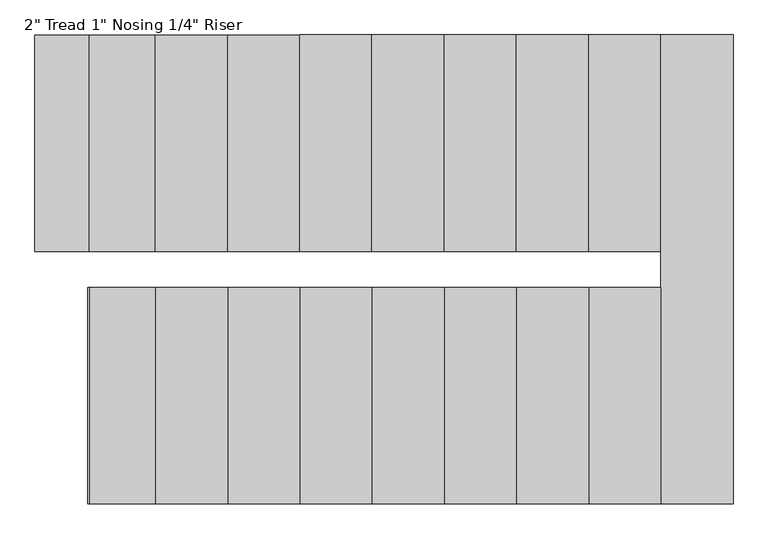
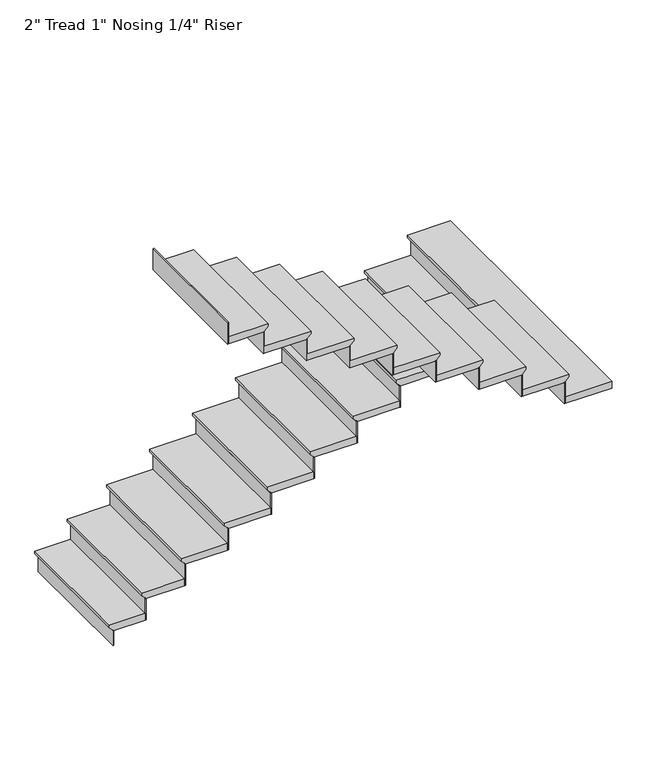
"""IFC4 building model written with IfcOpenShell, lengths in millimetres: stair flight geometry."""

from ifc_helpers import new_model, si_unit, origin, place, context, project, spatial, faceted_brep, source, transform, mapped, element, save


def stair_flight_3d163d7c(model_context):
    return source(origin(), model_context, "Body", "Brep", [
        faceted_brep([(8572.5, 8280.4, 3189.3710526), (8572.5, 8280.4, 3208.4210526), (8572.5, 9194.8, 3208.4210526), (8572.5, 9194.8, 3189.3710526), (8597.9, 8280.4, 3163.9710526), (8597.9, 9194.8, 3163.9710526), (8826.5, 8280.4, 3208.4210526), (8826.5, 9194.8, 3208.4210526), (8597.9, 9194.8, 3157.6210526), (8826.5, 9194.8, 3157.6210526), (8826.5, 8280.4, 3157.6210526), (8597.9, 8280.4, 3157.6210526)], [[[0, 1, 2, 3]], [[4, 0, 3, 5]], [[2, 1, 6, 7]], [[8, 9, 10, 11]], [[2, 7, 9, 8, 5, 3]], [[8, 11, 4, 5]], [[6, 1, 0, 4, 11, 10]], [[7, 6, 10, 9]]]),
        faceted_brep([(8597.9, 8280.4, 3157.6210526), (8597.9, 8280.4, 3048.0), (8604.25, 8280.4, 3048.0), (8604.25, 8280.4, 3157.6210526), (8597.9, 9194.8, 3157.6210526), (8604.25, 9194.8, 3157.6210526), (8604.25, 9194.8, 3048.0), (8597.9, 9194.8, 3048.0)], [[[0, 1, 2, 3]], [[4, 5, 6, 7]], [[1, 0, 4, 7]], [[2, 1, 7, 6]], [[3, 2, 6, 5]], [[0, 3, 5, 4]]]),
        faceted_brep([(8826.5, 8280.4, 3318.0421053), (8826.5, 8280.4, 3157.6210526), (8832.85, 8280.4, 3157.6210526), (8832.85, 8280.4, 3318.0421053), (8826.5, 9194.8, 3318.0421053), (8832.85, 9194.8, 3318.0421053), (8832.85, 9194.8, 3157.6210526), (8826.5, 9194.8, 3157.6210526)], [[[0, 1, 2, 3]], [[4, 5, 6, 7]], [[1, 0, 4, 7]], [[2, 1, 7, 6]], [[3, 2, 6, 5]], [[0, 3, 5, 4]]]),
        faceted_brep([(8801.1, 9194.8, 3368.8421053), (8801.1, 8280.4, 3368.8421053), (9105.9, 8280.4, 3368.8421053), (9105.9, 9194.8, 3368.8421053), (8826.5, 9194.8, 3318.0421053), (9105.9, 9194.8, 3318.0421053), (9105.9, 8280.4, 3318.0421053), (8826.5, 8280.4, 3318.0421053), (8826.5, 9194.8, 3324.3921053), (8801.1, 9194.8, 3349.7921053), (8826.5, 8280.4, 3324.3921053), (8801.1, 8280.4, 3349.7921053)], [[[0, 1, 2, 3]], [[4, 5, 6, 7]], [[0, 3, 5, 4, 8, 9]], [[4, 7, 10, 8]], [[2, 1, 11, 10, 7, 6]], [[3, 2, 6, 5]], [[11, 1, 0, 9]], [[10, 11, 9, 8]]]),
        faceted_brep([(9105.9, 8280.4, 3478.4631579), (9105.9, 8280.4, 3318.0421053), (9112.25, 8280.4, 3318.0421053), (9112.25, 8280.4, 3478.4631579), (9105.9, 9194.8, 3478.4631579), (9112.25, 9194.8, 3478.4631579), (9112.25, 9194.8, 3318.0421053), (9105.9, 9194.8, 3318.0421053)], [[[0, 1, 2, 3]], [[4, 5, 6, 7]], [[1, 0, 4, 7]], [[2, 1, 7, 6]], [[3, 2, 6, 5]], [[0, 3, 5, 4]]]),
        faceted_brep([(9080.5, 9194.8, 3529.2631579), (9080.5, 8280.4, 3529.2631579), (9410.7, 8280.4, 3529.2631579), (9410.7, 9194.8, 3529.2631579), (9105.9, 9194.8, 3478.4631579), (9410.7, 9194.8, 3478.4631579), (9410.7, 8280.4, 3478.4631579), (9105.9, 8280.4, 3478.4631579), (9105.9, 9194.8, 3484.8131579), (9080.5, 9194.8, 3510.2131579), (9105.9, 8280.4, 3484.8131579), (9080.5, 8280.4, 3510.2131579)], [[[0, 1, 2, 3]], [[4, 5, 6, 7]], [[0, 3, 5, 4, 8, 9]], [[4, 7, 10, 8]], [[2, 1, 11, 10, 7, 6]], [[3, 2, 6, 5]], [[11, 1, 0, 9]], [[10, 11, 9, 8]]]),
        faceted_brep([(9410.7, 8280.4, 3638.8842105), (9410.7, 8280.4, 3478.4631579), (9417.05, 8280.4, 3478.4631579), (9417.05, 8280.4, 3638.8842105), (9410.7, 9194.8, 3638.8842105), (9417.05, 9194.8, 3638.8842105), (9417.05, 9194.8, 3478.4631579), (9410.7, 9194.8, 3478.4631579)], [[[0, 1, 2, 3]], [[4, 5, 6, 7]], [[1, 0, 4, 7]], [[2, 1, 7, 6]], [[3, 2, 6, 5]], [[0, 3, 5, 4]]]),
        faceted_brep([(9385.3, 9194.8, 3689.6842105), (9385.3, 8280.4, 3689.6842105), (9715.5, 8280.4, 3689.6842105), (9715.5, 9194.8, 3689.6842105), (9410.7, 9194.8, 3638.8842105), (9715.5, 9194.8, 3638.8842105), (9715.5, 8280.4, 3638.8842105), (9410.7, 8280.4, 3638.8842105), (9410.7, 9194.8, 3645.2342105), (9385.3, 9194.8, 3670.6342105), (9410.7, 8280.4, 3645.2342105), (9385.3, 8280.4, 3670.6342105)], [[[0, 1, 2, 3]], [[4, 5, 6, 7]], [[0, 3, 5, 4, 8, 9]], [[4, 7, 10, 8]], [[2, 1, 11, 10, 7, 6]], [[3, 2, 6, 5]], [[11, 1, 0, 9]], [[10, 11, 9, 8]]]),
        faceted_brep([(9715.5, 8280.4, 3799.3052632), (9715.5, 8280.4, 3638.8842105), (9721.85, 8280.4, 3638.8842105), (9721.85, 8280.4, 3799.3052632), (9715.5, 9194.8, 3799.3052632), (9721.85, 9194.8, 3799.3052632), (9721.85, 9194.8, 3638.8842105), (9715.5, 9194.8, 3638.8842105)], [[[0, 1, 2, 3]], [[4, 5, 6, 7]], [[1, 0, 4, 7]], [[2, 1, 7, 6]], [[3, 2, 6, 5]], [[0, 3, 5, 4]]]),
        faceted_brep([(9690.1, 9194.8, 3850.1052632), (9690.1, 8280.4, 3850.1052632), (10020.3, 8280.4, 3850.1052632), (10020.3, 9194.8, 3850.1052632), (9715.5, 9194.8, 3799.3052632), (10020.3, 9194.8, 3799.3052632), (10020.3, 8280.4, 3799.3052632), (9715.5, 8280.4, 3799.3052632), (9715.5, 9194.8, 3805.6552632), (9690.1, 9194.8, 3831.0552632), (9715.5, 8280.4, 3805.6552632), (9690.1, 8280.4, 3831.0552632)], [[[0, 1, 2, 3]], [[4, 5, 6, 7]], [[0, 3, 5, 4, 8, 9]], [[4, 7, 10, 8]], [[2, 1, 11, 10, 7, 6]], [[3, 2, 6, 5]], [[11, 1, 0, 9]], [[10, 11, 9, 8]]]),
        faceted_brep([(10020.3, 8280.4, 3959.7263158), (10020.3, 8280.4, 3799.3052632), (10026.65, 8280.4, 3799.3052632), (10026.65, 8280.4, 3959.7263158), (10020.3, 9194.8, 3959.7263158), (10026.65, 9194.8, 3959.7263158), (10026.65, 9194.8, 3799.3052632), (10020.3, 9194.8, 3799.3052632)], [[[0, 1, 2, 3]], [[4, 5, 6, 7]], [[1, 0, 4, 7]], [[2, 1, 7, 6]], [[3, 2, 6, 5]], [[0, 3, 5, 4]]]),
        faceted_brep([(9994.9, 9194.8, 4010.5263158), (9994.9, 8280.4, 4010.5263158), (10325.1, 8280.4, 4010.5263158), (10325.1, 9194.8, 4010.5263158), (10020.3, 9194.8, 3959.7263158), (10325.1, 9194.8, 3959.7263158), (10325.1, 8280.4, 3959.7263158), (10020.3, 8280.4, 3959.7263158), (10020.3, 9194.8, 3966.0763158), (9994.9, 9194.8, 3991.4763158), (10020.3, 8280.4, 3966.0763158), (9994.9, 8280.4, 3991.4763158)], [[[0, 1, 2, 3]], [[4, 5, 6, 7]], [[0, 3, 5, 4, 8, 9]], [[4, 7, 10, 8]], [[2, 1, 11, 10, 7, 6]], [[3, 2, 6, 5]], [[11, 1, 0, 9]], [[10, 11, 9, 8]]]),
        faceted_brep([(10325.1, 8280.4, 4120.1473684), (10325.1, 8280.4, 3959.7263158), (10331.45, 8280.4, 3959.7263158), (10331.45, 8280.4, 4120.1473684), (10325.1, 9194.8, 4120.1473684), (10331.45, 9194.8, 4120.1473684), (10331.45, 9194.8, 3959.7263158), (10325.1, 9194.8, 3959.7263158)], [[[0, 1, 2, 3]], [[4, 5, 6, 7]], [[1, 0, 4, 7]], [[2, 1, 7, 6]], [[3, 2, 6, 5]], [[0, 3, 5, 4]]]),
        faceted_brep([(10299.7, 9194.8, 4170.9473684), (10299.7, 8280.4, 4170.9473684), (10629.9, 8280.4, 4170.9473684), (10629.9, 9194.8, 4170.9473684), (10325.1, 9194.8, 4120.1473684), (10629.9, 9194.8, 4120.1473684), (10629.9, 8280.4, 4120.1473684), (10325.1, 8280.4, 4120.1473684), (10325.1, 9194.8, 4126.4973684), (10299.7, 9194.8, 4151.8973684), (10325.1, 8280.4, 4126.4973684), (10299.7, 8280.4, 4151.8973684)], [[[0, 1, 2, 3]], [[4, 5, 6, 7]], [[0, 3, 5, 4, 8, 9]], [[4, 7, 10, 8]], [[2, 1, 11, 10, 7, 6]], [[3, 2, 6, 5]], [[11, 1, 0, 9]], [[10, 11, 9, 8]]]),
        faceted_brep([(10629.9, 8280.4, 4280.5684211), (10629.9, 8280.4, 4120.1473684), (10636.25, 8280.4, 4120.1473684), (10636.25, 8280.4, 4280.5684211), (10629.9, 9194.8, 4280.5684211), (10636.25, 9194.8, 4280.5684211), (10636.25, 9194.8, 4120.1473684), (10629.9, 9194.8, 4120.1473684)], [[[0, 1, 2, 3]], [[4, 5, 6, 7]], [[1, 0, 4, 7]], [[2, 1, 7, 6]], [[3, 2, 6, 5]], [[0, 3, 5, 4]]]),
        faceted_brep([(10604.5, 9194.8, 4331.3684211), (10604.5, 8280.4, 4331.3684211), (10934.7, 8280.4, 4331.3684211), (10934.7, 9194.8, 4331.3684211), (10629.9, 9194.8, 4280.5684211), (10934.7, 9194.8, 4280.5684211), (10934.7, 8280.4, 4280.5684211), (10629.9, 8280.4, 4280.5684211), (10629.9, 9194.8, 4286.9184211), (10604.5, 9194.8, 4312.3184211), (10629.9, 8280.4, 4286.9184211), (10604.5, 8280.4, 4312.3184211)], [[[0, 1, 2, 3]], [[4, 5, 6, 7]], [[0, 3, 5, 4, 8, 9]], [[4, 7, 10, 8]], [[2, 1, 11, 10, 7, 6]], [[3, 2, 6, 5]], [[11, 1, 0, 9]], [[10, 11, 9, 8]]]),
        faceted_brep([(10934.7, 8280.4, 4440.9894737), (10934.7, 8280.4, 4280.5684211), (10941.05, 8280.4, 4280.5684211), (10941.05, 8280.4, 4440.9894737), (10934.7, 9194.8, 4440.9894737), (10941.05, 9194.8, 4440.9894737), (10941.05, 9194.8, 4280.5684211), (10934.7, 9194.8, 4280.5684211)], [[[0, 1, 2, 3]], [[4, 5, 6, 7]], [[1, 0, 4, 7]], [[2, 1, 7, 6]], [[3, 2, 6, 5]], [[0, 3, 5, 4]]]),
        faceted_brep([(10909.3, 9194.8, 4491.7894737), (10909.3, 8280.4, 4491.7894737), (11239.5, 8280.4, 4491.7894737), (11239.5, 9194.8, 4491.7894737), (10934.7, 9194.8, 4440.9894737), (11239.5, 9194.8, 4440.9894737), (11239.5, 8280.4, 4440.9894737), (10934.7, 8280.4, 4440.9894737), (10934.7, 9194.8, 4447.3394737), (10909.3, 9194.8, 4472.7394737), (10934.7, 8280.4, 4447.3394737), (10909.3, 8280.4, 4472.7394737)], [[[0, 1, 2, 3]], [[4, 5, 6, 7]], [[0, 3, 5, 4, 8, 9]], [[4, 7, 10, 8]], [[2, 1, 11, 10, 7, 6]], [[3, 2, 6, 5]], [[11, 1, 0, 9]], [[10, 11, 9, 8]]]),
        faceted_brep([(11239.5, 8280.4, 4601.4105263), (11239.5, 8280.4, 4440.9894737), (11245.85, 8280.4, 4440.9894737), (11245.85, 8280.4, 4601.4105263), (11239.5, 9194.8, 4601.4105263), (11245.85, 9194.8, 4601.4105263), (11245.85, 9194.8, 4440.9894737), (11239.5, 9194.8, 4440.9894737)], [[[0, 1, 2, 3]], [[4, 5, 6, 7]], [[1, 0, 4, 7]], [[2, 1, 7, 6]], [[3, 2, 6, 5]], [[0, 3, 5, 4]]]),
        faceted_brep([(11188.7, 7213.6, 4652.2105263), (11518.9, 7213.6, 4652.2105263), (11518.9, 9194.8, 4652.2105263), (11214.1, 9194.8, 4652.2105263), (11214.1, 8128.0, 4652.2105263), (11188.7, 8128.0, 4652.2105263), (11518.9, 7213.6, 4601.4105263), (11188.7, 7213.6, 4601.4105263), (11188.7, 8128.0, 4601.4105263), (11214.1, 8128.0, 4601.4105263), (11214.1, 8280.4, 4601.4105263), (11239.5, 8280.4, 4601.4105263), (11239.5, 9194.8, 4601.4105263), (11518.9, 9194.8, 4601.4105263), (11239.5, 9194.8, 4607.7605263), (11214.1, 9194.8, 4633.1605263), (11239.5, 8280.4, 4607.7605263), (11214.1, 8280.4, 4633.1605263)], [[[0, 1, 2, 3, 4, 5]], [[6, 7, 8, 9, 10, 11, 12, 13]], [[1, 0, 7, 6]], [[2, 1, 6, 13]], [[3, 2, 13, 12, 14, 15]], [[12, 11, 16, 14]], [[11, 10, 17, 16]], [[4, 3, 15, 17, 10, 9]], [[5, 4, 9, 8]], [[0, 5, 8, 7]], [[15, 14, 16, 17]]]),
        faceted_brep([(11188.7, 8128.0, 4761.8315789), (11188.7, 8128.0, 4601.4105263), (11182.35, 8128.0, 4601.4105263), (11182.35, 8128.0, 4761.8315789), (11188.7, 7213.6, 4761.8315789), (11182.35, 7213.6, 4761.8315789), (11182.35, 7213.6, 4601.4105263), (11188.7, 7213.6, 4601.4105263)], [[[0, 1, 2, 3]], [[4, 5, 6, 7]], [[1, 0, 4, 7]], [[2, 1, 7, 6]], [[3, 2, 6, 5]], [[0, 3, 5, 4]]]),
        faceted_brep([(11214.1, 7213.6, 4812.6315789), (11214.1, 8128.0, 4812.6315789), (10883.9, 8128.0, 4812.6315789), (10883.9, 7213.6, 4812.6315789), (11188.7, 7213.6, 4761.8315789), (10883.9, 7213.6, 4761.8315789), (10883.9, 8128.0, 4761.8315789), (11188.7, 8128.0, 4761.8315789), (11188.7, 7213.6, 4768.1815789), (11214.1, 7213.6, 4793.5815789), (11188.7, 8128.0, 4768.1815789), (11214.1, 8128.0, 4793.5815789)], [[[0, 1, 2, 3]], [[4, 5, 6, 7]], [[0, 3, 5, 4, 8, 9]], [[4, 7, 10, 8]], [[2, 1, 11, 10, 7, 6]], [[3, 2, 6, 5]], [[11, 1, 0, 9]], [[10, 11, 9, 8]]]),
        faceted_brep([(10883.9, 8128.0, 4922.2526316), (10883.9, 8128.0, 4761.8315789), (10877.55, 8128.0, 4761.8315789), (10877.55, 8128.0, 4922.2526316), (10883.9, 7213.6, 4922.2526316), (10877.55, 7213.6, 4922.2526316), (10877.55, 7213.6, 4761.8315789), (10883.9, 7213.6, 4761.8315789)], [[[0, 1, 2, 3]], [[4, 5, 6, 7]], [[1, 0, 4, 7]], [[2, 1, 7, 6]], [[3, 2, 6, 5]], [[0, 3, 5, 4]]]),
        faceted_brep([(10909.3, 7213.6, 4973.0526316), (10909.3, 8128.0, 4973.0526316), (10579.1, 8128.0, 4973.0526316), (10579.1, 7213.6, 4973.0526316), (10883.9, 7213.6, 4922.2526316), (10579.1, 7213.6, 4922.2526316), (10579.1, 8128.0, 4922.2526316), (10883.9, 8128.0, 4922.2526316), (10883.9, 7213.6, 4928.6026316), (10909.3, 7213.6, 4954.0026316), (10883.9, 8128.0, 4928.6026316), (10909.3, 8128.0, 4954.0026316)], [[[0, 1, 2, 3]], [[4, 5, 6, 7]], [[0, 3, 5, 4, 8, 9]], [[4, 7, 10, 8]], [[2, 1, 11, 10, 7, 6]], [[3, 2, 6, 5]], [[11, 1, 0, 9]], [[10, 11, 9, 8]]]),
        faceted_brep([(10579.1, 8128.0, 5082.6736842), (10579.1, 8128.0, 4922.2526316), (10572.75, 8128.0, 4922.2526316), (10572.75, 8128.0, 5082.6736842), (10579.1, 7213.6, 5082.6736842), (10572.75, 7213.6, 5082.6736842), (10572.75, 7213.6, 4922.2526316), (10579.1, 7213.6, 4922.2526316)], [[[0, 1, 2, 3]], [[4, 5, 6, 7]], [[1, 0, 4, 7]], [[2, 1, 7, 6]], [[3, 2, 6, 5]], [[0, 3, 5, 4]]]),
        faceted_brep([(10604.5, 7213.6, 5133.4736842), (10604.5, 8128.0, 5133.4736842), (10274.3, 8128.0, 5133.4736842), (10274.3, 7213.6, 5133.4736842), (10579.1, 7213.6, 5082.6736842), (10274.3, 7213.6, 5082.6736842), (10274.3, 8128.0, 5082.6736842), (10579.1, 8128.0, 5082.6736842), (10579.1, 7213.6, 5089.0236842), (10604.5, 7213.6, 5114.4236842), (10579.1, 8128.0, 5089.0236842), (10604.5, 8128.0, 5114.4236842)], [[[0, 1, 2, 3]], [[4, 5, 6, 7]], [[0, 3, 5, 4, 8, 9]], [[4, 7, 10, 8]], [[2, 1, 11, 10, 7, 6]], [[3, 2, 6, 5]], [[11, 1, 0, 9]], [[10, 11, 9, 8]]]),
        faceted_brep([(10274.3, 8128.0, 5243.0947368), (10274.3, 8128.0, 5082.6736842), (10267.95, 8128.0, 5082.6736842), (10267.95, 8128.0, 5243.0947368), (10274.3, 7213.6, 5243.0947368), (10267.95, 7213.6, 5243.0947368), (10267.95, 7213.6, 5082.6736842), (10274.3, 7213.6, 5082.6736842)], [[[0, 1, 2, 3]], [[4, 5, 6, 7]], [[1, 0, 4, 7]], [[2, 1, 7, 6]], [[3, 2, 6, 5]], [[0, 3, 5, 4]]]),
        faceted_brep([(10299.7, 7213.6, 5293.8947368), (10299.7, 8128.0, 5293.8947368), (9969.5, 8128.0, 5293.8947368), (9969.5, 7213.6, 5293.8947368), (10274.3, 7213.6, 5243.0947368), (9969.5, 7213.6, 5243.0947368), (9969.5, 8128.0, 5243.0947368), (10274.3, 8128.0, 5243.0947368), (10274.3, 7213.6, 5249.4447368), (10299.7, 7213.6, 5274.8447368), (10274.3, 8128.0, 5249.4447368), (10299.7, 8128.0, 5274.8447368)], [[[0, 1, 2, 3]], [[4, 5, 6, 7]], [[0, 3, 5, 4, 8, 9]], [[4, 7, 10, 8]], [[2, 1, 11, 10, 7, 6]], [[3, 2, 6, 5]], [[11, 1, 0, 9]], [[10, 11, 9, 8]]]),
        faceted_brep([(9969.5, 8128.0, 5403.5157895), (9969.5, 8128.0, 5243.0947368), (9963.15, 8128.0, 5243.0947368), (9963.15, 8128.0, 5403.5157895), (9969.5, 7213.6, 5403.5157895), (9963.15, 7213.6, 5403.5157895), (9963.15, 7213.6, 5243.0947368), (9969.5, 7213.6, 5243.0947368)], [[[0, 1, 2, 3]], [[4, 5, 6, 7]], [[1, 0, 4, 7]], [[2, 1, 7, 6]], [[3, 2, 6, 5]], [[0, 3, 5, 4]]]),
        faceted_brep([(9994.9, 7213.6, 5454.3157895), (9994.9, 8128.0, 5454.3157895), (9664.7, 8128.0, 5454.3157895), (9664.7, 7213.6, 5454.3157895), (9969.5, 7213.6, 5403.5157895), (9664.7, 7213.6, 5403.5157895), (9664.7, 8128.0, 5403.5157895), (9969.5, 8128.0, 5403.5157895), (9969.5, 7213.6, 5409.8657895), (9994.9, 7213.6, 5435.2657895), (9969.5, 8128.0, 5409.8657895), (9994.9, 8128.0, 5435.2657895)], [[[0, 1, 2, 3]], [[4, 5, 6, 7]], [[0, 3, 5, 4, 8, 9]], [[4, 7, 10, 8]], [[2, 1, 11, 10, 7, 6]], [[3, 2, 6, 5]], [[11, 1, 0, 9]], [[10, 11, 9, 8]]]),
        faceted_brep([(9664.7, 8128.0, 5563.9368421), (9664.7, 8128.0, 5403.5157895), (9658.35, 8128.0, 5403.5157895), (9658.35, 8128.0, 5563.9368421), (9664.7, 7213.6, 5563.9368421), (9658.35, 7213.6, 5563.9368421), (9658.35, 7213.6, 5403.5157895), (9664.7, 7213.6, 5403.5157895)], [[[0, 1, 2, 3]], [[4, 5, 6, 7]], [[1, 0, 4, 7]], [[2, 1, 7, 6]], [[3, 2, 6, 5]], [[0, 3, 5, 4]]]),
        faceted_brep([(9690.1, 7213.6, 5614.7368421), (9690.1, 8128.0, 5614.7368421), (9359.9, 8128.0, 5614.7368421), (9359.9, 7213.6, 5614.7368421), (9664.7, 7213.6, 5563.9368421), (9359.9, 7213.6, 5563.9368421), (9359.9, 8128.0, 5563.9368421), (9664.7, 8128.0, 5563.9368421), (9664.7, 7213.6, 5570.2868421), (9690.1, 7213.6, 5595.6868421), (9664.7, 8128.0, 5570.2868421), (9690.1, 8128.0, 5595.6868421)], [[[0, 1, 2, 3]], [[4, 5, 6, 7]], [[0, 3, 5, 4, 8, 9]], [[4, 7, 10, 8]], [[2, 1, 11, 10, 7, 6]], [[3, 2, 6, 5]], [[11, 1, 0, 9]], [[10, 11, 9, 8]]]),
        faceted_brep([(9359.9, 8128.0, 5724.3578947), (9359.9, 8128.0, 5563.9368421), (9353.55, 8128.0, 5563.9368421), (9353.55, 8128.0, 5724.3578947), (9359.9, 7213.6, 5724.3578947), (9353.55, 7213.6, 5724.3578947), (9353.55, 7213.6, 5563.9368421), (9359.9, 7213.6, 5563.9368421)], [[[0, 1, 2, 3]], [[4, 5, 6, 7]], [[1, 0, 4, 7]], [[2, 1, 7, 6]], [[3, 2, 6, 5]], [[0, 3, 5, 4]]]),
        faceted_brep([(9385.3, 7213.6, 5775.1578947), (9385.3, 8128.0, 5775.1578947), (9055.1, 8128.0, 5775.1578947), (9055.1, 7213.6, 5775.1578947), (9359.9, 7213.6, 5724.3578947), (9055.1, 7213.6, 5724.3578947), (9055.1, 8128.0, 5724.3578947), (9359.9, 8128.0, 5724.3578947), (9359.9, 7213.6, 5730.7078947), (9385.3, 7213.6, 5756.1078947), (9359.9, 8128.0, 5730.7078947), (9385.3, 8128.0, 5756.1078947)], [[[0, 1, 2, 3]], [[4, 5, 6, 7]], [[0, 3, 5, 4, 8, 9]], [[4, 7, 10, 8]], [[2, 1, 11, 10, 7, 6]], [[3, 2, 6, 5]], [[11, 1, 0, 9]], [[10, 11, 9, 8]]]),
        faceted_brep([(9055.1, 8128.0, 5884.7789474), (9055.1, 8128.0, 5724.3578947), (9048.75, 8128.0, 5724.3578947), (9048.75, 8128.0, 5884.7789474), (9055.1, 7213.6, 5884.7789474), (9048.75, 7213.6, 5884.7789474), (9048.75, 7213.6, 5724.3578947), (9055.1, 7213.6, 5724.3578947)], [[[0, 1, 2, 3]], [[4, 5, 6, 7]], [[1, 0, 4, 7]], [[2, 1, 7, 6]], [[3, 2, 6, 5]], [[0, 3, 5, 4]]]),
        faceted_brep([(8801.1, 8128.0, 6045.2), (8801.1, 8128.0, 5884.7789474), (8794.75, 8128.0, 5884.7789474), (8794.75, 8128.0, 6045.2), (8801.1, 7213.6, 6045.2), (8794.75, 7213.6, 6045.2), (8794.75, 7213.6, 5884.7789474), (8801.1, 7213.6, 5884.7789474)], [[[0, 1, 2, 3]], [[4, 5, 6, 7]], [[1, 0, 4, 7]], [[2, 1, 7, 6]], [[3, 2, 6, 5]], [[0, 3, 5, 4]]]),
        faceted_brep([(9080.5, 7213.6, 5935.5789474), (9080.5, 8128.0, 5935.5789474), (8801.1, 8128.0, 5935.5789474), (8801.1, 7213.6, 5935.5789474), (9055.1, 7213.6, 5884.7789474), (8801.1, 7213.6, 5884.7789474), (8801.1, 8128.0, 5884.7789474), (9055.1, 8128.0, 5884.7789474), (9055.1, 7213.6, 5891.1289474), (9080.5, 7213.6, 5916.5289474), (9055.1, 8128.0, 5891.1289474), (9080.5, 8128.0, 5916.5289474)], [[[0, 1, 2, 3]], [[4, 5, 6, 7]], [[0, 3, 5, 4, 8, 9]], [[4, 7, 10, 8]], [[2, 1, 11, 10, 7, 6]], [[3, 2, 6, 5]], [[11, 1, 0, 9]], [[10, 11, 9, 8]]]),
    ])


if __name__ == "__main__":
    model = new_model("IFC4")
    model_context = context("Model", 3, world=origin())
    ifc_project = project(units=[si_unit("LENGTHUNIT", "METRE", prefix="MILLI")], contexts=[model_context])
    site = spatial("IfcSite", under=ifc_project)
    building = spatial("IfcBuilding", under=site)
    placement = place(None, origin())
    stair_flight_shape = stair_flight_3d163d7c(model_context)
    element("IfcStairFlight", 1, ObjectType="2\" Tread 1\" Nosing 1/4\" Riser", at=placement, inside=building, context=model_context, shape_type="MappedRepresentation", body=[
        mapped(stair_flight_shape, transform((0.0, 0.0, 0.0), x_axis=(1.0, 0.0, 0.0), y_axis=(0.0, 1.0, 0.0), z_axis=(0.0, 0.0, 1.0))),
    ])
    save(model, "model.ifc")
